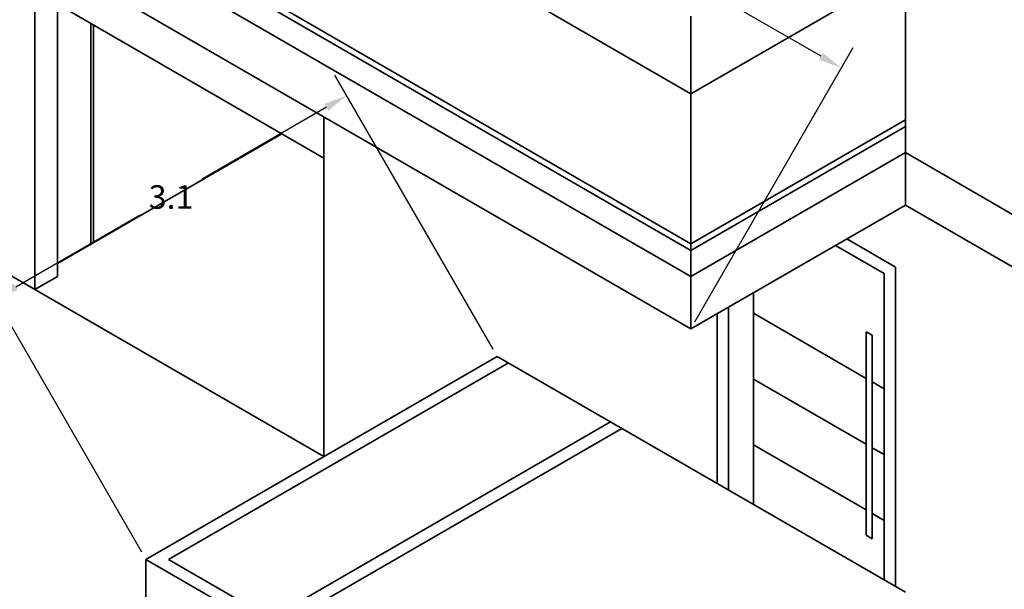
# Model space of a CAD drawing. Units: metres. Extents: x 12735 to 25554, y 20954 to 41989.
# Tile 5 of 15: x 12748.612 to 12756.135, y 20970.327 to 20974.676. Entities that reach past the tile are written whole.
import ezdxf

# ---------------------------------------------------------------- set-up
doc = ezdxf.new("R2010")
doc.units = ezdxf.units.M
doc.layers.get('Defpoints').update_dxf_attribs({"lineweight": 13})
doc.layers.add('A-ANNO-DIMS', color=2, linetype='Continuous', lineweight=18)
doc.layers.add('A-ELEV', color=7, linetype='Continuous', lineweight=35)
doc.styles.get("Standard").update_dxf_attribs({"font": 'arial.ttf'})
doc.dimstyles.get("Standard").update_dxf_attribs({"dimtxt": 0.18, "dimasz": 0.18, "dimexe": 0.18, "dimexo": 0.0625, "dimgap": 0.09, "dimtad": 0, "dimtih": 1, "dimtoh": 1, "dimdec": 4, "dimzin": 0, "dimdsep": 46, "dimtxsty": 'Standard', "dimcen": 0.09, "dimadec": 0, "dimazin": 0, "dimtfac": 1, "dimtdec": 4, "dimtofl": 0, "dimtmove": 0, "dimatfit": 3, "dimfxl": 1, "dimtolj": 1, "dimtzin": 0, "dimarcsym": 0})

# ---------------------------------------------------------------- blocks, each defined once
blk = doc.blocks.new('*D9')
at = {"layer": 'A-ANNO-DIMS', "color": 0, "lineweight": -2, "transparency": 16777216}
for p, q in [((12781.0041, 20970.8701), (12781.0041, 20953.8934)), ((12737.8426, 20966.671), (12737.8426, 20953.8934)), ((12738.0226, 20954.0734), (12759.0261, 20954.0734)), ((12780.8241, 20954.0734), (12759.8206, 20954.0734))]:
    blk.add_line(p, q, dxfattribs=at)
at = {"layer": 'A-ANNO-DIMS', "color": 0, "transparency": 16777216}
for points in [[(12738.0226, 20954.1034), (12738.0226, 20954.0434), (12737.8426, 20954.0734)], [(12780.8241, 20954.1034), (12780.8241, 20954.0434), (12781.0041, 20954.0734)]]:
    blk.add_solid(points, dxfattribs=at)
at = {"layer": 'Defpoints', "color": 0, "transparency": 16777216}
for p in [(12781.0041, 20970.9326), (12737.8426, 20966.7335), (12781.0041, 20954.0734)]:
    blk.add_point(p, dxfattribs=at)
at = {"layer": 'A-ANNO-DIMS', "color": 0, "transparency": 16777216, "insert": (12759.4234, 20954.0734), "char_height": 0.18, "attachment_point": 5}
blk.add_mtext('\\A1;43.16', dxfattribs=at)
blk = doc.blocks.new('*D10')
at = {"layer": 'A-ANNO-DIMS', "color": 0, "lineweight": -2, "transparency": 16777216}
for p, q in [((12766.6445, 20994.8247), (12783.4841, 20994.8247)), ((12783.3041, 20994.6447), (12783.3041, 20975.781)), ((12783.3041, 20956.5534), (12783.3041, 20975.4171)), ((12755.8494, 20956.3734), (12783.4841, 20956.3734))]:
    blk.add_line(p, q, dxfattribs=at)
at = {"layer": 'A-ANNO-DIMS', "color": 0, "transparency": 16777216}
for points in [[(12783.2741, 20994.6447), (12783.3341, 20994.6447), (12783.3041, 20994.8247)], [(12783.2741, 20956.5534), (12783.3341, 20956.5534), (12783.3041, 20956.3734)]]:
    blk.add_solid(points, dxfattribs=at)
at = {"layer": 'Defpoints', "color": 0, "transparency": 16777216}
for p in [(12766.582, 20994.8247), (12783.3041, 20994.8247), (12755.7869, 20956.3734)]:
    blk.add_point(p, dxfattribs=at)
at = {"layer": 'A-ANNO-DIMS', "color": 0, "transparency": 16777216, "insert": (12783.3041, 20975.599), "char_height": 0.18, "attachment_point": 5}
blk.add_mtext('\\A1;38.45', dxfattribs=at)
blk = doc.blocks.new('*D12')
at = {"layer": 'A-ANNO-DIMS', "color": 0, "lineweight": -2, "transparency": 16777216}
for p, q in [((12781.0354, 20970.8785), (12782.2441, 20968.7848)), ((12781.9983, 20968.8507), (12769.8606, 20961.843)), ((12757.0927, 20954.4715), (12769.2304, 20961.4792)), ((12755.8181, 20956.3192), (12757.0269, 20954.2256))]:
    blk.add_line(p, q, dxfattribs=at)
at = {"layer": 'A-ANNO-DIMS', "color": 0, "transparency": 16777216}
for points in [[(12781.9833, 20968.8767), (12782.0133, 20968.8247), (12782.1541, 20968.9407)], [(12757.0777, 20954.4975), (12757.1077, 20954.4455), (12756.9369, 20954.3815)]]:
    blk.add_solid(points, dxfattribs=at)
at = {"layer": 'Defpoints', "color": 0, "transparency": 16777216}
for p in [(12781.0041, 20970.9326), (12755.7869, 20956.3734), (12756.9369, 20954.3815)]:
    blk.add_point(p, dxfattribs=at)
at = {"layer": 'A-ANNO-DIMS', "color": 0, "transparency": 16777216, "insert": (12769.5455, 20961.6611), "char_height": 0.18, "attachment_point": 5}
blk.add_mtext('\\A1;29.12', dxfattribs=at)
blk = doc.blocks.new('*D21')
at = {"layer": 'A-ANNO-DIMS', "color": 0, "lineweight": -2, "transparency": 16777216}
for p, q in [((12747.3609, 20976.0704), (12748.5697, 20978.164)), ((12748.6355, 20977.9181), (12751.3698, 20976.3395)), ((12754.7343, 20974.397), (12752, 20975.9757)), ((12753.7714, 20972.3693), (12754.9802, 20974.4629))]:
    blk.add_line(p, q, dxfattribs=at)
at = {"layer": 'A-ANNO-DIMS', "color": 0, "transparency": 16777216}
for points in [[(12748.6505, 20977.9441), (12748.6205, 20977.8922), (12748.4797, 20978.0081)], [(12754.7493, 20974.423), (12754.7193, 20974.371), (12754.8902, 20974.307)]]:
    blk.add_solid(points, dxfattribs=at)
at = {"layer": 'Defpoints', "color": 0, "transparency": 16777216}
for p in [(12747.3297, 20976.0163), (12754.8902, 20974.307), (12753.7402, 20972.3152)]:
    blk.add_point(p, dxfattribs=at)
at = {"layer": 'A-ANNO-DIMS', "color": 0, "transparency": 16777216, "insert": (12751.6849, 20976.1576), "char_height": 0.18, "attachment_point": 5}
blk.add_mtext('\\A1;7.402', dxfattribs=at)
blk = doc.blocks.new('*D26')
at = {"layer": 'A-ANNO-DIMS', "color": 0, "lineweight": -2, "transparency": 16777216}
for p, q in [((12752.23, 20972.1598), (12751.0213, 20974.2535)), ((12750.9554, 20974.0076), (12750.0053, 20973.4591)), ((12748.5825, 20972.6376), (12749.5325, 20973.1861)), ((12749.5453, 20970.6098), (12748.3366, 20972.7035))]:
    blk.add_line(p, q, dxfattribs=at)
at = {"layer": 'A-ANNO-DIMS', "color": 0, "transparency": 16777216}
for points in [[(12750.9404, 20974.0335), (12750.9704, 20973.9816), (12751.1113, 20974.0976)], [(12748.5675, 20972.6635), (12748.5975, 20972.6116), (12748.4266, 20972.5476)]]:
    blk.add_solid(points, dxfattribs=at)
at = {"layer": 'Defpoints', "color": 0, "transparency": 16777216}
for p in [(12751.1113, 20974.0976), (12752.2613, 20972.1057), (12749.5766, 20970.5557)]:
    blk.add_point(p, dxfattribs=at)
at = {"layer": 'A-ANNO-DIMS', "color": 0, "transparency": 16777216, "insert": (12749.7689, 20973.3226), "char_height": 0.18, "attachment_point": 5}
blk.add_mtext('\\A1;3.1', dxfattribs=at)

msp = doc.modelspace()

# ---------------------------------------------------------------- linework, layer by layer
at = {"layer": 'A-ELEV'}
for p, q in [((12755.379, 20979.1473), (12755.379, 20973.2613)), ((12747.6761, 20977.6118), (12753.7402, 20974.1107)), ((12753.7402, 20972.9652), (12747.6761, 20976.4663)), ((12753.7402, 20972.9152), (12747.6761, 20976.4163)), ((12753.7402, 20972.7152), (12747.6761, 20976.2163)), ((12753.7402, 20972.3152), (12747.3297, 20976.0163)), ((12748.7281, 20975.2089), (12748.7281, 20972.6165)), ((12748.9013, 20975.1089), (12748.9013, 20972.7165)), ((12753.7402, 20974.1107), (12755.379, 20975.0569)), ((12750.937, 20973.6198), (12748.9013, 20974.7951)), ((12749.1549, 20974.6487), (12749.1549, 20972.9622)), ((12749.1771, 20974.6358), (12749.1771, 20972.9751)), ((12753.7402, 20972.3152), (12753.7402, 20974.7041)), ((12750.937, 20971.3411), (12750.937, 20973.9336)), ((12755.379, 20973.9113), (12753.7402, 20972.9652)), ((12748.9013, 20972.8159), (12750.6154, 20973.8055)), ((12755.379, 20973.8613), (12753.7402, 20972.9152)), ((12755.379, 20973.6613), (12753.7402, 20972.7152)), ((12757.8038, 20972.2613), (12755.379, 20973.6613)), ((12755.379, 20973.2613), (12753.7402, 20972.3152)), ((12760.2287, 20970.4613), (12755.379, 20973.2613)), ((12754.9316, 20973.003), (12755.3044, 20972.7878)), ((12750.937, 20971.3411), (12748.1844, 20972.9304)), ((12754.845, 20972.953), (12755.2178, 20972.7378)), ((12755.3044, 20972.7878), (12755.3044, 20970.3488)), ((12748.7281, 20972.6165), (12748.9013, 20972.7165)), ((12755.2178, 20972.7378), (12755.2178, 20970.3988)), ((12754.2178, 20972.5909), (12754.2178, 20970.9761)), ((12754.0271, 20972.4808), (12754.0271, 20971.0862)), ((12753.9405, 20972.4308), (12753.9405, 20971.1362)), ((12754.2178, 20972.4351), (12755.0794, 20971.9377)), ((12755.0794, 20972.2937), (12755.1255, 20972.267)), ((12755.0794, 20970.7403), (12755.0794, 20972.2937)), ((12755.1255, 20972.267), (12755.1255, 20970.7136)), ((12749.5766, 20970.5557), (12752.2613, 20972.1057)), ((12755.379, 20970.3057), (12752.2613, 20972.1057)), ((12749.7498, 20970.5557), (12752.3479, 20972.0557)), ((12754.2178, 20971.9327), (12755.0794, 20971.4353)), ((12755.1255, 20971.911), (12755.2178, 20971.8577)), ((12750.5292, 20970.1057), (12753.1273, 20971.6057)), ((12750.5292, 20970.0057), (12753.2139, 20971.5557)), ((12754.2178, 20971.4303), (12755.0794, 20970.9329)), ((12755.1255, 20971.4086), (12755.2178, 20971.3554)), ((12755.1255, 20970.9063), (12755.2178, 20970.853)), ((12755.1255, 20970.7136), (12755.0794, 20970.7403)), ((12750.5292, 20970.0057), (12749.5766, 20970.5557)), ((12749.5766, 20969.7557), (12749.5766, 20970.5557)), ((12750.5292, 20970.1057), (12749.7498, 20970.5557))]:
    msp.add_line(p, q, dxfattribs=at)
at = {"layer": 'Defpoints'}
for p in [(12754.2178, 20972.4351), (12754.2178, 20971.9327), (12754.2178, 20971.4303)]:
    msp.add_point(p, dxfattribs=at)

# ---------------------------------------------------------------- dimensions: what is measured, and where the dimension line sits
at = {"layer": 'A-ANNO-DIMS'}
for base, p1, p2, angle, override, picture, middle in [((12783.3041, 20994.8247), (12755.7869, 20956.3734), (12766.582, 20994.8247), 90, {"dimdec": 2, "dimlfac": 1, "dimrnd": 0, "dimzin": 0, "dimdsep": 46, "dimlunit": 2}, '*D10', (12783.3041, 20975.599)), ((12754.8902, 20974.307), (12747.3297, 20976.0163), (12753.7402, 20972.3152), 330, {"dimdec": 3, "dimlfac": 1, "dimrnd": 0, "dimzin": 0, "dimdsep": 46, "dimlunit": 2}, '*D21', (12751.6849, 20976.1576)), ((12751.1113, 20974.0976), (12749.5766, 20970.5557), (12752.2613, 20972.1057), 30, {"dimdec": 1, "dimlfac": 1, "dimrnd": 0, "dimzin": 0, "dimdsep": 46, "dimlunit": 2}, '*D26', (12749.7689, 20973.3226)), ((12756.9369, 20954.3815), (12781.0041, 20970.9326), (12755.7869, 20956.3734), 210, {"dimdec": 2, "dimlfac": 1, "dimrnd": 0, "dimzin": 0, "dimdsep": 46, "dimlunit": 2}, '*D12', (12769.5455, 20961.6611))]:
    dim = msp.add_linear_dim(base=base, p1=p1, p2=p2, angle=angle, dimstyle='Standard', override=override, dxfattribs=at)
    dim.commit()
    dim.dimension.update_dxf_attribs({"geometry": picture, "text_midpoint": middle})
dim = msp.add_linear_dim(base=(12781.0041, 20954.0734), p1=(12737.8426, 20966.7335), p2=(12781.0041, 20970.9326), dimstyle='Standard', override={"dimdec": 2, "dimlfac": 1, "dimrnd": 0, "dimzin": 0, "dimdsep": 46, "dimlunit": 2}, dxfattribs=at)
dim.commit()
dim.dimension.update_dxf_attribs({"geometry": '*D9', "text_midpoint": (12759.4234, 20954.0734)})

doc.saveas('drawing.dxf')
